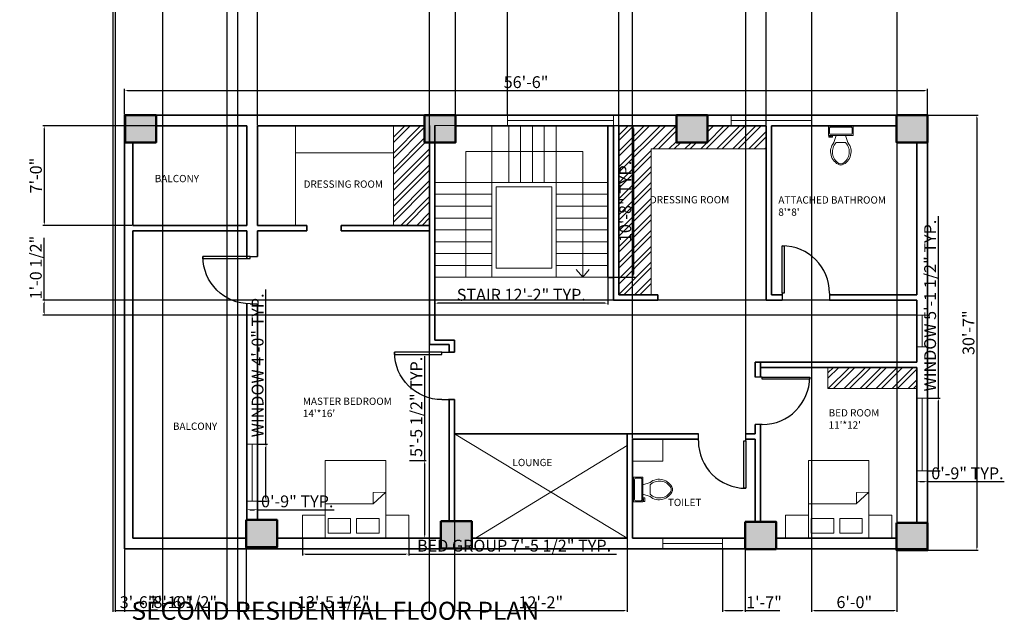
# Model space of a CAD drawing. Units: inches. Extents: x 1964 to 3462, y 1879 to 2909.
# Tile 2 of 4: x 2631 to 3462, y 1879 to 2387. Entities that reach past the tile are written whole.
import ezdxf

# ---------------------------------------------------------------- set-up
doc = ezdxf.new("R2010")
doc.units = ezdxf.units.IN
for name, color, linetype, lineweight in [('A-ANNO-DIMS', 2, 'Continuous', 18), ('A-ANNO-TEXT', 7, 'Continuous', 35), ('A-AREA-IDEN', 7, 'Continuous', 18), ('A-COLS', 1, 'Continuous', 50), ('A-COLS-PATT', 252, 'Continuous', 13), ('A-DOOR', 4, 'Continuous', 25), ('A-FLOR-CASE', 9, 'Continuous', 18), ('A-FLOR-FIXT', 4, 'Continuous', 18), ('A-FLOR-OPEN', 8, 'Continuous', 13), ('A-FLOR-PATT', 252, 'Continuous', 13), ('A-FLOR-STRS', 3, 'Continuous', 18), ('A-FURN', 8, 'Continuous', 18), ('A-GLAZ', 4, 'Continuous', 18), ('A-WALL', 7, 'Continuous', 35)]:
    doc.layers.add(name, color=color, linetype=linetype, lineweight=lineweight)
doc.styles.get("Standard").update_dxf_attribs({"font": 'arial.ttf'})
doc.dimstyles.new('ISO-25', dxfattribs={"dimtxt": 10, "dimasz": 2.5, "dimexe": 1.25, "dimexo": 0.625, "dimtad": 1, "dimdec": 0, "dimlunit": 4, "dimtxsty": 'Standard', "dimcen": 2.5, "dimadec": 0, "dimazin": 0, "dimtfac": 1, "dimtdec": 0, "dimtmove": 0, "dimatfit": 3, "dimfxl": 1, "dimarcsym": 0})

# ---------------------------------------------------------------- blocks, each defined once
blk = doc.blocks.new('*U2')
for p, q in [((0, 0), (0, -6)), ((40, 0), (40, -6))]:
    blk.add_line(p, q)
blk.add_lwpolyline([(0, 0), (0, 40), (1.75, 40), (1.75, 0)], close=True)
blk.add_arc((0, 0), 40, 0, 90)
blk = doc.blocks.new('*U6')
for p, q in [((-8, -8.5), (-8, -8)), ((-7, -8), (-7, -9.5)), ((-4, -8), (-6, -14)), ((4, -8), (6, -14)), ((9.5, -6), (9.5, -2)), ((-10, -8.5), (-8, -8.5)), ((-10, -9.5), (-10, -8.5)), ((-7, -9.5), (-10, -9.5)), ((4, -14), (-4, -14))]:
    blk.add_line(p, q)
blk.add_lwpolyline([(10.5, -8), (10.5, 0), (-10.5, 0), (-10.5, -8)], close=True)
for points in [[(-9.5, -2), (-9.5, -6)], [(8.5, -1), (-8.5, -1)], [(-8.5, -7), (8.5, -7)]]:
    blk.add_lwpolyline(points)
for centre, radius, start, end in [((-8.62, -1.88), 0.884, 81.8699, 188.1301), ((-8.62, -6.12), 0.884, 171.8699, 278.1301), ((8.62, -1.88), 0.884, 351.8699, 98.1301), ((8.62, -6.12), 0.884, 261.8699, 8.1301), ((3.52, -21.58), 12.17, 141.46911, 247.97143), ((4.2, -21.82), 11.33, 136.36773, 238.94682), ((-3.52, -21.58), 12.17, 292.02843, 38.53071), ((-4.2, -21.82), 11.33, 301.05301, 43.63209), ((0, -27.88), 4, 245.73182, 294.26817), ((0, -29), 4, 254.86053, 285.13947)]:
    blk.add_arc(centre, radius, start, end)
blk = doc.blocks.new('*D11')
at = {"layer": 'A-ANNO-DIMS', "color": 0, "lineweight": -2, "transparency": 16777216}
for p, q in [((2719.86, 2307.2), (2719.86, 2328.6)), ((2722.36, 2327.35), (3395.05, 2327.35)), ((3397.55, 2307.2), (3397.55, 2328.6))]:
    blk.add_line(p, q, dxfattribs=at)
at = {"layer": 'A-ANNO-DIMS', "color": 0, "lineweight": 100, "transparency": 16777216}
for points in [[(2722.36, 2327.76), (2722.36, 2326.93), (2719.86, 2327.35)], [(3395.05, 2327.76), (3395.05, 2326.93), (3397.55, 2327.35)]]:
    blk.add_solid(points, dxfattribs=at)
at = {"layer": 'Defpoints', "color": 0, "lineweight": 100, "transparency": 16777216}
for p in [(3397.55, 2327.35), (2719.86, 2306.57), (3397.55, 2306.57)]:
    blk.add_point(p, dxfattribs=at)
at = {"layer": 'A-ANNO-DIMS', "color": 0, "transparency": 16777216, "insert": (3058.71, 2333.08), "char_height": 10, "attachment_point": 5}
blk.add_mtext('56\'-6"', dxfattribs=at)
blk = doc.blocks.new('*D12')
at = {"layer": 'A-ANNO-DIMS', "color": 0, "lineweight": -2, "transparency": 16777216}
for p, q in [((3398.18, 2306.57), (3440.34, 2306.57)), ((3439.09, 2304.07), (3439.09, 1941.77)), ((3398.18, 1939.27), (3440.34, 1939.27))]:
    blk.add_line(p, q, dxfattribs=at)
at = {"layer": 'A-ANNO-DIMS', "color": 0, "lineweight": 100, "transparency": 16777216}
for points in [[(3438.67, 2304.07), (3439.5, 2304.07), (3439.09, 2306.57)], [(3438.67, 1941.77), (3439.5, 1941.77), (3439.09, 1939.27)]]:
    blk.add_solid(points, dxfattribs=at)
at = {"layer": 'Defpoints', "color": 0, "lineweight": 100, "transparency": 16777216}
for p in [(3397.55, 2306.57), (3397.55, 1939.27), (3439.09, 1939.27)]:
    blk.add_point(p, dxfattribs=at)
at = {"layer": 'A-ANNO-DIMS', "color": 0, "transparency": 16777216, "insert": (3433.35, 2122.92), "char_height": 10, "attachment_point": 5, "rotation": 90}
blk.add_mtext('30\'-7"', dxfattribs=at)
blk = doc.blocks.new('COL-RECT-26x23')
blk.add_lwpolyline([(0, 23.08), (26.15, 23.08), (26.15, 0), (0, 0)], close=True)
blk = doc.blocks.new('BED-DOUBLE-WITH-NIGHTSTANDS')
for p, q in [((59.67, 28.98), (70.38, 38.71)), ((70.38, 38.71), (59.8, 38.58)), ((59.8, 38.58), (59.8, 29.09)), ((19.34, 28.98), (59.67, 28.98))]:
    blk.add_line(p, q)
for points in [[(19.34, 0), (70.38, 0), (70.38, 65.5), (19.34, 65.5)], [(19.34, 0), (0, 0), (0, 19.34), (19.34, 19.34)], [(89.72, 0), (70.38, 0), (70.38, 19.34), (89.72, 19.34)], [(21.67, 4.3), (40.69, 4.3), (40.69, 16.59), (21.67, 16.59)], [(45.74, 4.3), (64.76, 4.3), (64.76, 16.59), (45.74, 16.59)]]:
    blk.add_lwpolyline(points, close=True)
blk = doc.blocks.new('STAIR-RETURN-RESIDENTIAL')
for p, q in [((0, 128), (145.76, 128)), ((21.08, 128), (15.66, 121.5)), ((21.08, 21.87), (21.08, 128)), ((21.08, 128), (26.5, 121.5)), ((43.5, 124.05), (43.5, 128)), ((97.76, 128), (97.76, 118)), ((119.78, 128), (119.78, 21.87)), ((0, 118), (43.5, 118)), ((43.5, 48), (43.5, 124.05)), ((47.14, 51.64), (47.14, 120.41)), ((47.14, 120.41), (94.12, 120.41)), ((94.12, 51.64), (94.12, 120.41)), ((97.76, 48), (97.76, 124.05)), ((97.76, 118), (145.76, 118)), ((0, 108), (43.5, 108)), ((97.76, 108), (145.76, 108)), ((0, 98), (43.5, 98)), ((97.76, 98), (145.76, 98)), ((0, 88), (43.5, 88)), ((97.76, 88), (145.76, 88)), ((0, 78), (43.5, 78)), ((97.76, 78), (145.76, 78)), ((0, 68), (43.5, 68)), ((97.76, 68), (145.76, 68)), ((0, 58), (43.5, 58)), ((94.12, 51.64), (47.14, 51.64)), ((97.76, 58), (145.76, 58)), ((97.76, 50.18), (97.76, 0)), ((0, 48), (145.76, 48)), ((97.76, 48), (43.5, 48)), ((43.5, 48), (43.5, 0)), ((53.5, 48), (53.5, 0)), ((63.5, 48), (63.5, 0)), ((73.5, 48), (73.5, 0)), ((83.5, 48), (83.5, 0)), ((119.78, 21.87), (21.08, 21.87))]:
    blk.add_line(p, q)
blk = doc.blocks.new('WIN-48IN')
blk.add_line((4.5, 0), (4.5, 48.18))
blk.add_lwpolyline([(0, 0), (9, 0), (9, 48.18), (0, 48.18)], close=True)
blk = doc.blocks.new('WIN-50IN')
blk.add_line((0, 4.5), (50.22, 4.5))
blk.add_lwpolyline([(0, 9), (50.22, 9), (50.22, 0), (0, 0)], close=True)
blk = doc.blocks.new('WIN-61IN')
blk.add_line((4.5, 61.35), (4.5, 0))
blk.add_lwpolyline([(0, 61.35), (9, 61.35), (9, 0), (0, 0)], close=True)
blk = doc.blocks.new('WIN-27IN')
blk.add_line((4.5, 26.51), (4.5, 0))
blk.add_lwpolyline([(0, 0), (9, 0), (9, 26.51), (0, 26.51)], close=True)
blk = doc.blocks.new('WIN-90IN')
blk.add_line((0, 4.5), (89.57, 4.5))
blk.add_lwpolyline([(0, 9), (89.57, 9), (89.57, 0), (0, 0)], close=True)
blk = doc.blocks.new('*D29')
at = {"layer": 'A-ANNO-DIMS', "color": 0, "lineweight": -2, "transparency": 16777216}
for p, q in [((2870.02, 1948.95), (2870.02, 1934.86)), ((2959.73, 1948.95), (2959.73, 1934.86)), ((2872.52, 1936.11), (2957.23, 1936.11)), ((2959.73, 1936.11), (3135.01, 1936.11))]:
    blk.add_line(p, q, dxfattribs=at)
at = {"layer": 'A-ANNO-DIMS', "color": 0, "lineweight": 100, "transparency": 16777216}
for points in [[(2872.52, 1936.53), (2872.52, 1935.7), (2870.02, 1936.11)], [(2957.23, 1936.53), (2957.23, 1935.7), (2959.73, 1936.11)]]:
    blk.add_solid(points, dxfattribs=at)
at = {"layer": 'Defpoints', "color": 0, "lineweight": 100, "transparency": 16777216}
for p in [(2870.02, 1949.57), (2959.73, 1949.57), (2959.73, 1936.11)]:
    blk.add_point(p, dxfattribs=at)
at = {"layer": 'A-ANNO-DIMS', "color": 0, "transparency": 16777216, "insert": (3048.62, 1941.91), "char_height": 10, "attachment_point": 5}
blk.add_mtext('BED GROUP 7\'-5 1/2" TYP.', dxfattribs=at)
blk = doc.blocks.new('*D30')
at = {"layer": 'A-ANNO-DIMS', "color": 0, "lineweight": -2, "transparency": 16777216}
for p, q in [((2973.19, 2015.07), (2973.19, 2103.08)), ((2960.36, 2015.07), (2974.44, 2015.07)), ((2973.19, 1952.07), (2973.19, 2012.57)), ((2960.36, 1949.57), (2974.44, 1949.57))]:
    blk.add_line(p, q, dxfattribs=at)
at = {"layer": 'A-ANNO-DIMS', "color": 0, "lineweight": 100, "transparency": 16777216}
for points in [[(2972.77, 2012.57), (2973.61, 2012.57), (2973.19, 2015.07)], [(2972.77, 1952.07), (2973.61, 1952.07), (2973.19, 1949.57)]]:
    blk.add_solid(points, dxfattribs=at)
at = {"layer": 'Defpoints', "color": 0, "lineweight": 100, "transparency": 16777216}
for p in [(2959.73, 2015.07), (2973.19, 2015.07), (2959.73, 1949.57)]:
    blk.add_point(p, dxfattribs=at)
at = {"layer": 'A-ANNO-DIMS', "color": 0, "transparency": 16777216, "insert": (2967.39, 2060.33), "char_height": 10, "attachment_point": 5, "rotation": 90}
blk.add_mtext('5\'-5 1/2" TYP.', dxfattribs=at)
blk = doc.blocks.new('*D31')
at = {"layer": 'A-ANNO-DIMS', "color": 0, "lineweight": -2, "transparency": 16777216}
for p, q in [((2981.84, 2169.09), (2981.84, 2146.6)), ((3127.6, 2169.09), (3127.6, 2146.6)), ((3125.1, 2147.85), (2984.34, 2147.85))]:
    blk.add_line(p, q, dxfattribs=at)
at = {"layer": 'A-ANNO-DIMS', "color": 0, "lineweight": 100, "transparency": 16777216}
for points in [[(2984.34, 2148.27), (2984.34, 2147.43), (2981.84, 2147.85)], [(3125.1, 2148.27), (3125.1, 2147.43), (3127.6, 2147.85)]]:
    blk.add_solid(points, dxfattribs=at)
at = {"layer": 'Defpoints', "color": 0, "lineweight": 100, "transparency": 16777216}
for p in [(2981.84, 2169.71), (3127.6, 2169.71), (2981.84, 2147.85)]:
    blk.add_point(p, dxfattribs=at)
at = {"layer": 'A-ANNO-DIMS', "color": 0, "transparency": 16777216, "insert": (3054.72, 2153.65), "char_height": 10, "attachment_point": 5}
blk.add_mtext('STAIR 12\'-2" TYP.', dxfattribs=at)
blk = doc.blocks.new('*D32')
at = {"layer": 'A-ANNO-DIMS', "color": 0, "lineweight": -2, "transparency": 16777216}
for p, q in [((3128.22, 2297.71), (3150.71, 2297.71)), ((3149.46, 2295.21), (3149.46, 2172.21)), ((3128.22, 2169.71), (3150.71, 2169.71))]:
    blk.add_line(p, q, dxfattribs=at)
at = {"layer": 'A-ANNO-DIMS', "color": 0, "lineweight": 100, "transparency": 16777216}
for points in [[(3149.05, 2295.21), (3149.88, 2295.21), (3149.46, 2297.71)], [(3149.05, 2172.21), (3149.88, 2172.21), (3149.46, 2169.71)]]:
    blk.add_solid(points, dxfattribs=at)
at = {"layer": 'Defpoints', "color": 0, "lineweight": 100, "transparency": 16777216}
for p in [(3127.6, 2297.71), (3127.6, 2169.71), (3149.46, 2169.71)]:
    blk.add_point(p, dxfattribs=at)
at = {"layer": 'A-ANNO-DIMS', "color": 0, "transparency": 16777216, "insert": (3143.73, 2233.71), "char_height": 10, "attachment_point": 5, "rotation": 90}
blk.add_mtext('10\'-8" TYP.', dxfattribs=at)
blk = doc.blocks.new('*D33')
at = {"layer": 'A-ANNO-DIMS', "color": 0, "lineweight": -2, "transparency": 16777216}
for p, q in [((2839.29, 2028.96), (2839.29, 2159.25)), ((2832.69, 2028.96), (2840.54, 2028.96)), ((2839.29, 1983.28), (2839.29, 2026.46)), ((2832.69, 1980.78), (2840.54, 1980.78))]:
    blk.add_line(p, q, dxfattribs=at)
at = {"layer": 'A-ANNO-DIMS', "color": 0, "lineweight": 100, "transparency": 16777216}
for points in [[(2838.88, 2026.46), (2839.71, 2026.46), (2839.29, 2028.96)], [(2838.88, 1983.28), (2839.71, 1983.28), (2839.29, 1980.78)]]:
    blk.add_solid(points, dxfattribs=at)
at = {"layer": 'Defpoints', "color": 0, "lineweight": 100, "transparency": 16777216}
for p in [(2832.07, 2028.96), (2839.29, 2028.96), (2832.07, 1980.78)]:
    blk.add_point(p, dxfattribs=at)
at = {"layer": 'A-ANNO-DIMS', "color": 0, "transparency": 16777216, "insert": (2833.49, 2095.36), "char_height": 10, "attachment_point": 5, "rotation": 90}
blk.add_mtext('WINDOW 4\'-0" TYP.', dxfattribs=at)
blk = doc.blocks.new('*D34')
at = {"layer": 'A-ANNO-DIMS', "color": 0, "lineweight": -2, "transparency": 16777216}
for p, q in [((2823.07, 1980.15), (2823.07, 1972.3)), ((2832.07, 1980.15), (2832.07, 1972.3)), ((2825.57, 1973.55), (2829.57, 1973.55)), ((2832.07, 1973.55), (2896.77, 1973.55))]:
    blk.add_line(p, q, dxfattribs=at)
at = {"layer": 'A-ANNO-DIMS', "color": 0, "lineweight": 100, "transparency": 16777216}
for points in [[(2825.57, 1973.97), (2825.57, 1973.13), (2823.07, 1973.55)], [(2829.57, 1973.97), (2829.57, 1973.13), (2832.07, 1973.55)]]:
    blk.add_solid(points, dxfattribs=at)
at = {"layer": 'Defpoints', "color": 0, "lineweight": 100, "transparency": 16777216}
for p in [(2823.07, 1980.78), (2832.07, 1980.78), (2832.07, 1973.55)]:
    blk.add_point(p, dxfattribs=at)
at = {"layer": 'A-ANNO-DIMS', "color": 0, "transparency": 16777216, "insert": (2865.67, 1979.28), "char_height": 10, "attachment_point": 5}
blk.add_mtext('0\'-9" TYP.', dxfattribs=at)
blk = doc.blocks.new('*D37')
at = {"layer": 'A-ANNO-DIMS', "color": 0, "lineweight": -2, "transparency": 16777216}
for p, q in [((3406.76, 2067.79), (3406.76, 2221.38)), ((3398.18, 2067.79), (3408.01, 2067.79)), ((3406.76, 2008.94), (3406.76, 2065.29)), ((3398.18, 2006.44), (3408.01, 2006.44))]:
    blk.add_line(p, q, dxfattribs=at)
at = {"layer": 'A-ANNO-DIMS', "color": 0, "lineweight": 100, "transparency": 16777216}
for points in [[(3406.34, 2065.29), (3407.17, 2065.29), (3406.76, 2067.79)], [(3406.34, 2008.94), (3407.17, 2008.94), (3406.76, 2006.44)]]:
    blk.add_solid(points, dxfattribs=at)
at = {"layer": 'Defpoints', "color": 0, "lineweight": 100, "transparency": 16777216}
for p in [(3397.55, 2067.79), (3406.76, 2067.79), (3397.55, 2006.44)]:
    blk.add_point(p, dxfattribs=at)
at = {"layer": 'A-ANNO-DIMS', "color": 0, "transparency": 16777216, "insert": (3400.96, 2145.83), "char_height": 10, "attachment_point": 5, "rotation": 90}
blk.add_mtext('WINDOW 5\'-1 1/2" TYP.', dxfattribs=at)
blk = doc.blocks.new('*D38')
at = {"layer": 'A-ANNO-DIMS', "color": 0, "lineweight": -2, "transparency": 16777216}
for p, q in [((3388.55, 2005.81), (3388.55, 1995.98)), ((3397.55, 2005.81), (3397.55, 1995.98)), ((3391.05, 1997.23), (3395.05, 1997.23)), ((3397.55, 1997.23), (3462.26, 1997.23))]:
    blk.add_line(p, q, dxfattribs=at)
at = {"layer": 'A-ANNO-DIMS', "color": 0, "lineweight": 100, "transparency": 16777216}
for points in [[(3391.05, 1997.65), (3391.05, 1996.82), (3388.55, 1997.23)], [(3395.05, 1997.65), (3395.05, 1996.82), (3397.55, 1997.23)]]:
    blk.add_solid(points, dxfattribs=at)
at = {"layer": 'Defpoints', "color": 0, "lineweight": 100, "transparency": 16777216}
for p in [(3388.55, 2006.44), (3397.55, 2006.44), (3397.55, 1997.23)]:
    blk.add_point(p, dxfattribs=at)
at = {"layer": 'A-ANNO-DIMS', "color": 0, "transparency": 16777216, "insert": (3431.16, 2002.96), "char_height": 10, "attachment_point": 5}
blk.add_mtext('0\'-9" TYP.', dxfattribs=at)
blk = doc.blocks.new('*D53')
at = {"layer": 'A-ANNO-DIMS', "color": 0, "lineweight": -2, "transparency": 16777216}
for p, q in [((2709.93, 2826.73), (2709.93, 1887.22)), ((2751.91, 2826.73), (2751.91, 1887.22)), ((2712.43, 1888.47), (2749.41, 1888.47))]:
    blk.add_line(p, q, dxfattribs=at)
at = {"layer": 'A-ANNO-DIMS', "color": 0, "lineweight": 100, "transparency": 16777216}
for points in [[(2712.43, 1888.89), (2712.43, 1888.06), (2709.93, 1888.47)], [(2749.41, 1888.89), (2749.41, 1888.06), (2751.91, 1888.47)]]:
    blk.add_solid(points, dxfattribs=at)
at = {"layer": 'Defpoints', "color": 0, "lineweight": 100, "transparency": 16777216}
for p in [(2709.93, 2827.36), (2751.91, 2827.36), (2751.91, 1888.47)]:
    blk.add_point(p, dxfattribs=at)
at = {"layer": 'A-ANNO-DIMS', "color": 0, "transparency": 16777216, "insert": (2730.92, 1894.21), "char_height": 10, "attachment_point": 5}
blk.add_mtext('3\'-6"', dxfattribs=at)
blk = doc.blocks.new('*D56')
at = {"layer": 'A-ANNO-DIMS', "color": 0, "lineweight": -2, "transparency": 16777216}
for p, q in [((3299.67, 2687.56), (3299.67, 1887.22)), ((3371.67, 2687.56), (3371.67, 1887.22)), ((3302.17, 1888.47), (3369.17, 1888.47))]:
    blk.add_line(p, q, dxfattribs=at)
at = {"layer": 'A-ANNO-DIMS', "color": 0, "lineweight": 100, "transparency": 16777216}
for points in [[(3302.17, 1888.89), (3302.17, 1888.06), (3299.67, 1888.47)], [(3369.17, 1888.89), (3369.17, 1888.06), (3371.67, 1888.47)]]:
    blk.add_solid(points, dxfattribs=at)
at = {"layer": 'Defpoints', "color": 0, "lineweight": 100, "transparency": 16777216}
for p in [(3299.67, 2688.18), (3371.67, 2688.18), (3371.67, 1888.47)]:
    blk.add_point(p, dxfattribs=at)
at = {"layer": 'A-ANNO-DIMS', "color": 0, "transparency": 16777216, "insert": (3335.67, 1894.2), "char_height": 10, "attachment_point": 5}
blk.add_mtext('6\'-0"', dxfattribs=at)
blk = doc.blocks.new('*D57')
at = {"layer": 'A-ANNO-DIMS', "color": 0, "lineweight": -2, "transparency": 16777216}
for p, q in [((2711.98, 2582.23), (2711.98, 1887.22)), ((2806.18, 2582.23), (2806.18, 1887.22)), ((2714.48, 1888.47), (2803.68, 1888.47))]:
    blk.add_line(p, q, dxfattribs=at)
at = {"layer": 'A-ANNO-DIMS', "color": 0, "lineweight": 100, "transparency": 16777216}
for points in [[(2714.48, 1888.89), (2714.48, 1888.06), (2711.98, 1888.47)], [(2803.68, 1888.89), (2803.68, 1888.06), (2806.18, 1888.47)]]:
    blk.add_solid(points, dxfattribs=at)
at = {"layer": 'Defpoints', "color": 0, "lineweight": 100, "transparency": 16777216}
for p in [(2711.98, 2582.86), (2806.18, 2582.86), (2806.18, 1888.47)]:
    blk.add_point(p, dxfattribs=at)
at = {"layer": 'A-ANNO-DIMS', "color": 0, "transparency": 16777216, "insert": (2759.08, 1894.2), "char_height": 10, "attachment_point": 5}
blk.add_mtext('7\'-10"', dxfattribs=at)
blk = doc.blocks.new('*D58')
at = {"layer": 'A-ANNO-DIMS', "color": 0, "lineweight": -2, "transparency": 16777216}
for p, q in [((2815.18, 2582.23), (2815.18, 1887.22)), ((2976.91, 2582.23), (2976.91, 1887.22)), ((2817.68, 1888.47), (2974.41, 1888.47))]:
    blk.add_line(p, q, dxfattribs=at)
at = {"layer": 'A-ANNO-DIMS', "color": 0, "lineweight": 100, "transparency": 16777216}
for points in [[(2817.68, 1888.89), (2817.68, 1888.06), (2815.18, 1888.47)], [(2974.41, 1888.89), (2974.41, 1888.06), (2976.91, 1888.47)]]:
    blk.add_solid(points, dxfattribs=at)
at = {"layer": 'Defpoints', "color": 0, "lineweight": 100, "transparency": 16777216}
for p in [(2815.18, 2582.86), (2976.91, 2582.86), (2976.91, 1888.47)]:
    blk.add_point(p, dxfattribs=at)
at = {"layer": 'A-ANNO-DIMS', "color": 0, "transparency": 16777216, "insert": (2896.05, 1894.27), "char_height": 10, "attachment_point": 5}
blk.add_mtext('13\'-5 1/2"', dxfattribs=at)
blk = doc.blocks.new('*D62')
at = {"layer": 'A-ANNO-DIMS', "color": 0, "lineweight": -2, "transparency": 16777216}
for p, q in [((2719.86, 1939.95), (2719.86, 1887.22)), ((2822.51, 1941.17), (2822.51, 1887.22)), ((2722.36, 1888.47), (2820.01, 1888.47))]:
    blk.add_line(p, q, dxfattribs=at)
at = {"layer": 'A-ANNO-DIMS', "color": 0, "lineweight": 100, "transparency": 16777216}
for points in [[(2722.36, 1888.89), (2722.36, 1888.06), (2719.86, 1888.47)], [(2820.01, 1888.89), (2820.01, 1888.06), (2822.51, 1888.47)]]:
    blk.add_solid(points, dxfattribs=at)
at = {"layer": 'Defpoints', "color": 0, "lineweight": 100, "transparency": 16777216}
for p in [(2719.86, 1940.57), (2822.51, 1941.79), (2822.51, 1888.47)]:
    blk.add_point(p, dxfattribs=at)
at = {"layer": 'A-ANNO-DIMS', "color": 0, "transparency": 16777216, "insert": (2771.18, 1894.27), "char_height": 10, "attachment_point": 5}
blk.add_mtext('8\'-6 1/2"', dxfattribs=at)
blk = doc.blocks.new('*D63')
at = {"layer": 'A-ANNO-DIMS', "color": 0, "lineweight": -2, "transparency": 16777216}
for p, q in [((2745.94, 2297.57), (2650.93, 2297.57)), ((2652.18, 2295.07), (2652.18, 2215.99)), ((2726.19, 2213.49), (2650.93, 2213.49))]:
    blk.add_line(p, q, dxfattribs=at)
at = {"layer": 'A-ANNO-DIMS', "color": 0, "lineweight": 100, "transparency": 16777216}
for points in [[(2651.76, 2295.07), (2652.59, 2295.07), (2652.18, 2297.57)], [(2651.76, 2215.99), (2652.59, 2215.99), (2652.18, 2213.49)]]:
    blk.add_solid(points, dxfattribs=at)
at = {"layer": 'Defpoints', "color": 0, "lineweight": 100, "transparency": 16777216}
for p in [(2746.57, 2297.57), (2652.18, 2213.49), (2726.81, 2213.49)]:
    blk.add_point(p, dxfattribs=at)
at = {"layer": 'A-ANNO-DIMS', "color": 0, "transparency": 16777216, "insert": (2646.45, 2255.53), "char_height": 10, "attachment_point": 5, "rotation": 90}
blk.add_mtext('7\'-0"', dxfattribs=at)
blk = doc.blocks.new('*D64')
at = {"layer": 'A-ANNO-DIMS', "color": 0, "lineweight": -2, "transparency": 16777216}
for p, q in [((2832.07, 2298.2), (2832.07, 2889.94)), ((2834.57, 2888.69), (2974.84, 2888.69)), ((2977.34, 2298.34), (2977.34, 2889.94))]:
    blk.add_line(p, q, dxfattribs=at)
at = {"layer": 'A-ANNO-DIMS', "color": 0, "lineweight": 100, "transparency": 16777216}
for points in [[(2834.57, 2889.1), (2834.57, 2888.27), (2832.07, 2888.69)], [(2974.84, 2889.1), (2974.84, 2888.27), (2977.34, 2888.69)]]:
    blk.add_solid(points, dxfattribs=at)
at = {"layer": 'Defpoints', "color": 0, "lineweight": 100, "transparency": 16777216}
for p in [(2977.34, 2888.69), (2832.07, 2297.57), (2977.34, 2297.71)]:
    blk.add_point(p, dxfattribs=at)
at = {"layer": 'A-ANNO-DIMS', "color": 0, "transparency": 16777216, "insert": (2904.7, 2894.48), "char_height": 10, "attachment_point": 5}
blk.add_mtext('12\'-1 1/2"', dxfattribs=at)
blk = doc.blocks.new('*D65')
at = {"layer": 'A-ANNO-DIMS', "color": 0, "lineweight": -2, "transparency": 16777216}
for p, q in [((3137.07, 2298.2), (3137.07, 2889.94)), ((3139.57, 2888.69), (3258.77, 2888.69)), ((3261.27, 2298.2), (3261.27, 2889.94))]:
    blk.add_line(p, q, dxfattribs=at)
at = {"layer": 'A-ANNO-DIMS', "color": 0, "lineweight": 100, "transparency": 16777216}
for points in [[(3139.57, 2889.1), (3139.57, 2888.27), (3137.07, 2888.69)], [(3258.77, 2889.1), (3258.77, 2888.27), (3261.27, 2888.69)]]:
    blk.add_solid(points, dxfattribs=at)
at = {"layer": 'Defpoints', "color": 0, "lineweight": 100, "transparency": 16777216}
for p in [(3261.27, 2888.69), (3137.07, 2297.57), (3261.27, 2297.57)]:
    blk.add_point(p, dxfattribs=at)
at = {"layer": 'A-ANNO-DIMS', "color": 0, "transparency": 16777216, "insert": (3199.17, 2894.42), "char_height": 10, "attachment_point": 5}
blk.add_mtext('10\'-4"', dxfattribs=at)
blk = doc.blocks.new('*D66')
at = {"layer": 'A-ANNO-DIMS', "color": 0, "lineweight": -2, "transparency": 16777216}
for p, q in [((2998.29, 2037), (2998.29, 1887.22)), ((3144.05, 2037), (3144.05, 1887.22)), ((3000.79, 1888.47), (3141.55, 1888.47))]:
    blk.add_line(p, q, dxfattribs=at)
at = {"layer": 'A-ANNO-DIMS', "color": 0, "lineweight": 100, "transparency": 16777216}
for points in [[(3000.79, 1888.89), (3000.79, 1888.06), (2998.29, 1888.47)], [(3141.55, 1888.89), (3141.55, 1888.06), (3144.05, 1888.47)]]:
    blk.add_solid(points, dxfattribs=at)
at = {"layer": 'Defpoints', "color": 0, "lineweight": 100, "transparency": 16777216}
for p in [(2998.29, 2037.62), (3144.05, 2037.62), (3144.05, 1888.47)]:
    blk.add_point(p, dxfattribs=at)
at = {"layer": 'A-ANNO-DIMS', "color": 0, "transparency": 16777216, "insert": (3071.17, 1894.12), "char_height": 10, "attachment_point": 5}
blk.add_mtext('12\'-2"', dxfattribs=at)
blk = doc.blocks.new('*D67')
at = {"layer": 'A-ANNO-DIMS', "color": 0, "lineweight": -2, "transparency": 16777216}
for p, q in [((3148.55, 2033.75), (3148.55, 2889.94)), ((3151.05, 2888.69), (3241.63, 2888.69)), ((3244.13, 2034), (3244.13, 2889.94))]:
    blk.add_line(p, q, dxfattribs=at)
at = {"layer": 'A-ANNO-DIMS', "color": 0, "lineweight": 100, "transparency": 16777216}
for points in [[(3151.05, 2889.1), (3151.05, 2888.27), (3148.55, 2888.69)], [(3241.63, 2889.1), (3241.63, 2888.27), (3244.13, 2888.69)]]:
    blk.add_solid(points, dxfattribs=at)
at = {"layer": 'Defpoints', "color": 0, "lineweight": 100, "transparency": 16777216}
for p in [(3244.13, 2888.69), (3148.55, 2033.12), (3244.13, 2033.37)]:
    blk.add_point(p, dxfattribs=at)
at = {"layer": 'A-ANNO-DIMS', "color": 0, "transparency": 16777216, "insert": (3196.34, 2894.48), "char_height": 10, "attachment_point": 5}
blk.add_mtext('7\'-11 1/2"', dxfattribs=at)
blk = doc.blocks.new('*D68')
at = {"layer": 'A-ANNO-DIMS', "color": 0, "lineweight": -2, "transparency": 16777216}
for p, q in [((2999.25, 2307.2), (2999.25, 2889.94)), ((3001.75, 2888.69), (3040.51, 2888.69)), ((3043.01, 2307.2), (3043.01, 2889.94))]:
    blk.add_line(p, q, dxfattribs=at)
at = {"layer": 'A-ANNO-DIMS', "color": 0, "lineweight": 100, "transparency": 16777216}
for points in [[(3001.75, 2889.1), (3001.75, 2888.27), (2999.25, 2888.69)], [(3040.51, 2889.1), (3040.51, 2888.27), (3043.01, 2888.69)]]:
    blk.add_solid(points, dxfattribs=at)
at = {"layer": 'Defpoints', "color": 0, "lineweight": 100, "transparency": 16777216}
for p in [(3043.01, 2888.69), (2999.25, 2306.57), (3043.01, 2306.57)]:
    blk.add_point(p, dxfattribs=at)
at = {"layer": 'A-ANNO-DIMS', "color": 0, "transparency": 16777216, "insert": (3021.13, 2894.42), "char_height": 10, "attachment_point": 5}
blk.add_mtext('3\'-8"', dxfattribs=at)
blk = doc.blocks.new('*D69')
at = {"layer": 'A-ANNO-DIMS', "color": 0, "lineweight": -2, "transparency": 16777216}
for p, q in [((3224.47, 1939.95), (3224.47, 1887.22)), ((3243.55, 1939.66), (3243.55, 1887.22)), ((3226.97, 1888.47), (3241.05, 1888.47)), ((3243.55, 1888.47), (3272.95, 1888.47))]:
    blk.add_line(p, q, dxfattribs=at)
at = {"layer": 'A-ANNO-DIMS', "color": 0, "lineweight": 100, "transparency": 16777216}
for points in [[(3226.97, 1888.89), (3226.97, 1888.06), (3224.47, 1888.47)], [(3241.05, 1888.89), (3241.05, 1888.06), (3243.55, 1888.47)]]:
    blk.add_solid(points, dxfattribs=at)
at = {"layer": 'Defpoints', "color": 0, "lineweight": 100, "transparency": 16777216}
for p in [(3224.47, 1940.57), (3243.55, 1940.29), (3243.55, 1888.47)]:
    blk.add_point(p, dxfattribs=at)
at = {"layer": 'A-ANNO-DIMS', "color": 0, "transparency": 16777216, "insert": (3259.5, 1894.12), "char_height": 10, "attachment_point": 5}
blk.add_mtext('1\'-7"', dxfattribs=at)
blk = doc.blocks.new('*D70')
at = {"layer": 'A-ANNO-DIMS', "color": 0, "lineweight": -2, "transparency": 16777216}
for p, q in [((2652.18, 2150.28), (2652.18, 2202.98)), ((3387.93, 2150.28), (2650.93, 2150.28)), ((2652.18, 2140.1), (2652.18, 2147.78)), ((3387.93, 2137.6), (2650.93, 2137.6))]:
    blk.add_line(p, q, dxfattribs=at)
at = {"layer": 'A-ANNO-DIMS', "color": 0, "lineweight": 100, "transparency": 16777216}
for points in [[(2651.76, 2147.78), (2652.59, 2147.78), (2652.18, 2150.28)], [(2651.76, 2140.1), (2652.59, 2140.1), (2652.18, 2137.6)]]:
    blk.add_solid(points, dxfattribs=at)
at = {"layer": 'Defpoints', "color": 0, "lineweight": 100, "transparency": 16777216}
for p in [(2652.18, 2150.28), (3388.55, 2150.28), (3388.55, 2137.6)]:
    blk.add_point(p, dxfattribs=at)
at = {"layer": 'A-ANNO-DIMS', "color": 0, "transparency": 16777216, "insert": (2646.38, 2177.88), "char_height": 10, "attachment_point": 5, "rotation": 90}
blk.add_mtext('1\'-0 1/2"', dxfattribs=at)

msp = doc.modelspace()

# ---------------------------------------------------------------- hatches: boundary and pattern name
at = {"layer": 'A-COLS-PATT'}
h = msp.add_hatch(color=256, dxfattribs=at)
h.dxf.hatch_style = 1
h.paths.add_polyline_path([(3397.55, 2306.57), (3371.4, 2306.57), (3371.4, 2283.49), (3397.55, 2283.49)])
h.paths.add_polyline_path([(3211.73, 2306.57), (3185.58, 2306.57), (3185.58, 2297.57), (3185.79, 2297.57), (3185.79, 2283.49), (3211.73, 2283.49)])
h.paths.add_polyline_path([(2999.25, 2306.57), (2973.1, 2306.57), (2973.1, 2283.49), (2977.89, 2283.49)])
h.paths.add_polyline_path([(2999.25, 2306.57), (2977.89, 2283.49), (2998.29, 2283.49), (2999.25, 2283.49)], flags=17)
h.paths.add_polyline_path([(2746.57, 2306.57), (2720.41, 2306.57), (2745.76, 2283.49), (2746.57, 2283.49)])
h.paths.add_polyline_path([(2720.41, 2306.57), (2720.41, 2283.49), (2745.76, 2283.49)], flags=17)
h.paths.add_polyline_path([(2848.66, 1964.88), (2822.51, 1964.88), (2822.51, 1941.79), (2848.66, 1941.79)])
h.paths.add_polyline_path([(3012.86, 1963.84), (2986.71, 1963.84), (2986.71, 1940.76), (3012.86, 1940.76)])
h.paths.add_polyline_path([(3269.71, 1963.37), (3243.55, 1963.37), (3243.55, 1940.57), (3269.71, 1940.57)])
h.paths.add_polyline_path([(3397.55, 1962.36), (3371.4, 1962.36), (3371.4, 1940.57), (3397.55, 1940.57)])
at = {"layer": 'A-FLOR-PATT'}
h = msp.add_hatch(dxfattribs=at)
h.set_pattern_fill('ANSI32', color=256)
h.set_pattern_definition([(45, (161.698, 257.281), (-6.735192, 6.735192), []), (45, (166.188, 257.281), (-6.735192, 6.735192), [])])
h.paths.add_polyline_path([(3131.67, 2557.57), (3171.89, 2557.57), (3171.89, 2623.36), (3131.67, 2623.36)])
h.paths.add_polyline_path([(3164.38, 2278.1), (3261.27, 2278.1), (3261.27, 2297.57), (3231.68, 2297.57), (3211.73, 2297.57), (3211.73, 2283.49), (3185.58, 2283.49), (3185.58, 2297.57), (3166.29, 2297.57), (3142.29, 2297.57), (3137.07, 2297.57), (3137.07, 2154.78), (3164.38, 2154.78)])
h.paths.add_polyline_path([(2977.34, 2283.49), (2973.1, 2283.49), (2973.1, 2297.57), (2946.77, 2297.57), (2946.77, 2213.49), (2977.34, 2213.49)])
h.paths.add_polyline_path([(3313.48, 2093.57), (3313.48, 2075.7), (3388.55, 2075.7), (3388.55, 2093.57)])
h.paths.add_polyline_path([(3161.01, 2228.59), (3238.21, 2228.59), (3238.21, 2241.28), (3161.01, 2241.28)], flags=24)

# ---------------------------------------------------------------- linework, layer by layer
at = {"layer": 'A-COLS'}
for points in [[(2973.1, 2306.57), (2999.25, 2306.57), (2999.25, 2283.49), (2973.1, 2283.49)], [(3185.58, 2306.57), (3211.73, 2306.57), (3211.73, 2283.49), (3185.58, 2283.49)]]:
    msp.add_lwpolyline(points, close=True, dxfattribs=at)
at = {"layer": 'A-FLOR-CASE'}
for p, q in [((2864.22, 2213.49), (2864.22, 2297.57)), ((2946.77, 2213.49), (2946.77, 2297.57)), ((3164.38, 2154.78), (3164.38, 2278.1)), ((3164.38, 2278.1), (3261.27, 2278.1)), ((2864.22, 2274.77), (2946.77, 2274.77))]:
    msp.add_line(p, q, dxfattribs=at)
msp.add_lwpolyline([(3388.55, 2093.57), (3313.48, 2093.57), (3313.48, 2075.7), (3388.55, 2075.7)], close=True, dxfattribs=at)
at = {"layer": 'A-FLOR-FIXT'}
msp.add_lwpolyline([(3148.55, 2033.12), (3174.08, 2033.12), (3174.08, 2014.52), (3148.55, 2014.52)], close=True, dxfattribs=at)
at = {"layer": 'A-FLOR-OPEN'}
for p, q in [((3144.05, 1949.57), (2998.29, 2037.62)), ((3016.1, 1949.57), (3144.05, 2027.78))]:
    msp.add_line(p, q, dxfattribs=at)
at = {"layer": 'A-FLOR-STRS'}
for q in [(3017.84, 2297.71), (3017.84, 2297.71), (2981.84, 2261.71)]:
    msp.add_line((2981.84, 2297.71), q, dxfattribs=at)
at = {"layer": 'A-GLAZ'}
msp.add_line((3231.68, 2302.07), (3299.86, 2302.07), dxfattribs=at)
msp.add_lwpolyline([(3261.27, 2297.57), (3231.68, 2297.57), (3231.68, 2306.57), (3299.86, 2306.57), (3299.86, 2297.57), (3265.77, 2297.57)], dxfattribs=at)
at = {"layer": 'A-WALL'}
for p, q in [((2768.79, 2306.57), (2719.86, 2306.57)), ((2719.86, 2306.57), (2719.86, 2053.07)), ((2933.79, 2306.57), (2768.79, 2306.57)), ((3397.55, 2306.57), (3397.55, 1940.57)), ((2746.57, 2297.57), (2768.79, 2297.57)), ((2768.79, 2297.57), (2782.83, 2297.57)), ((2777.79, 2297.57), (2823.07, 2297.57)), ((2823.07, 2213.49), (2823.07, 2297.57)), ((2832.07, 2213.49), (2832.07, 2297.57)), ((2832.07, 2297.57), (2973.1, 2297.57)), ((2977.34, 2297.71), (2977.34, 2153.71)), ((2981.84, 2297.71), (2981.84, 2149.21)), ((2999.25, 2297.57), (3132.57, 2297.57)), ((3127.6, 2283.44), (3127.6, 2297.57)), ((3132.57, 2297.57), (3132.57, 2150.28)), ((3137.07, 2297.57), (3137.07, 2154.78)), ((3137.07, 2297.57), (3142.29, 2297.57)), ((3142.29, 2297.57), (3166.29, 2297.57)), ((3166.29, 2297.57), (3185.79, 2297.57)), ((3261.27, 2297.57), (3261.27, 2225.57)), ((3265.77, 2297.57), (3265.77, 2225.57)), ((3371.4, 2297.57), (3316.55, 2297.57)), ((2726.81, 2213.49), (2726.81, 2283.49)), ((3127.6, 2194.21), (3127.6, 2283.44)), ((3261.27, 2225.57), (3261.27, 2150.28)), ((3265.77, 2225.57), (3265.77, 2154.78)), ((2823.07, 2213.49), (2726.81, 2213.49)), ((2873.68, 2213.49), (2832.07, 2213.49)), ((2873.68, 2213.49), (2873.68, 2208.99)), ((2977.34, 2213.49), (2902.74, 2213.49)), ((2902.74, 2213.49), (2902.74, 2208.99)), ((2726.81, 2057.57), (2726.81, 2208.99)), ((2823.07, 2208.99), (2726.81, 2208.99)), ((2823.07, 2185.48), (2823.07, 2208.99)), ((2873.68, 2208.99), (2832.07, 2208.99)), ((2832.07, 2187.23), (2832.07, 2208.99)), ((2977.34, 2208.99), (2902.74, 2208.99)), ((3127.6, 2169.44), (3127.6, 2194.21)), ((3132.1, 2169.44), (3127.6, 2169.44)), ((3132.1, 2169.44), (3132.57, 2169.44)), ((2977.34, 2153.71), (2977.34, 2112.92)), ((3169.87, 2154.78), (3137.07, 2154.78)), ((3169.87, 2154.78), (3169.87, 2150.28)), ((3265.77, 2154.78), (3274.8, 2154.78)), ((3314.8, 2154.78), (3388.55, 2154.78)), ((2823.07, 2053.07), (2823.07, 2147.34)), ((2832.07, 2053.07), (2832.07, 2147.23)), ((2981.84, 2149.21), (2981.84, 2116.62)), ((3169.87, 2150.28), (3132.57, 2150.28)), ((3261.27, 2150.28), (3274.8, 2150.28)), ((3314.8, 2150.28), (3388.55, 2150.28)), ((2993.79, 2112.92), (2977.34, 2112.92)), ((2981.84, 2116.62), (2998.29, 2116.62)), ((2993.79, 2106.51), (2993.79, 2112.92)), ((2998.29, 2116.62), (2998.29, 2106.41)), ((2993.79, 2106.41), (2993.79, 2106.51)), ((2998.29, 2106.41), (2993.79, 2106.41)), ((3388.55, 2098.07), (3252.05, 2098.07)), ((3252.05, 2098.07), (3263.73, 2098.07)), ((3252.05, 2093.57), (3252.05, 2098.07)), ((3256.55, 2093.57), (3256.55, 2098.07)), ((3252.05, 2093.57), (3252.05, 2085.44)), ((3388.55, 2093.57), (3256.55, 2093.57)), ((3256.55, 2093.57), (3256.55, 2085.44)), ((3256.55, 2093.57), (3263.73, 2093.57)), ((3388.55, 1962.36), (3388.55, 2093.57)), ((2998.29, 2066.41), (2993.37, 2066.41)), ((2993.79, 2066.41), (2993.79, 2057.57)), ((2998.29, 2053.07), (2998.29, 2066.41)), ((2719.86, 2053.07), (2719.86, 1940.57)), ((2726.81, 2057.57), (2726.81, 1949.57)), ((2823.07, 2053.07), (2823.07, 1964.88)), ((2832.07, 2053.07), (2832.07, 1964.88)), ((2993.79, 2057.57), (2993.79, 1963.84)), ((2998.29, 2053.07), (2998.29, 1963.84)), ((3252.05, 2045.44), (3252.05, 2037.62)), ((3256.55, 2045.44), (3256.55, 1963.37)), ((3147.39, 2037.62), (2998.29, 2037.62)), ((3144.05, 2037.62), (3144.05, 2025.31)), ((3204.13, 2037.62), (3144.05, 2037.62)), ((3252.05, 2037.62), (3244.13, 2037.62)), ((3144.05, 1949.57), (3144.05, 2027.78)), ((3148.55, 1949.57), (3148.55, 2033.12)), ((3204.13, 2033.12), (3148.55, 2033.12)), ((3252.05, 2033.12), (3244.13, 2033.12)), ((3252.05, 2033.12), (3252.05, 1963.37)), ((3144.05, 1949.57), (3144.05, 1985.57)), ((2726.81, 1949.57), (2789.13, 1949.57)), ((3144.05, 1949.57), (3108.05, 1949.57)), ((3144.05, 1949.57), (3108.05, 1949.57)), ((3180.05, 1949.57), (3148.55, 1949.57)), ((3243.55, 1949.57), (3180.05, 1949.57)), ((2719.86, 1940.57), (2789.13, 1940.57)), ((2768.79, 1940.57), (2881.66, 1940.57))]:
    msp.add_line(p, q, dxfattribs=at)
for points in [[(2768.79, 2306.57), (3397.55, 2306.57), (3397.55, 1940.57), (2768.79, 1940.57)], [(3397.55, 2144.33), (3397.55, 2306.57), (2858.63, 2306.57)], [(2777.79, 2297.57), (2823.07, 2297.57)], [(2832.07, 2297.57), (2973.1, 2297.57)], [(2999.25, 2297.57), (3132.57, 2297.57)], [(3137.07, 2297.57), (3185.79, 2297.57)], [(3211.73, 2297.57), (3261.27, 2297.57)], [(3265.77, 2297.57), (3371.4, 2297.57)], [(3388.55, 2283.49), (3388.55, 2154.78)], [(3388.55, 2150.28), (3388.55, 2098.07)], [(2858.63, 1940.57), (3397.55, 1940.57), (3397.55, 2104.33)], [(3388.55, 2093.57), (3388.55, 1962.36)], [(2823.07, 1949.57), (2777.79, 1949.57)], [(2986.71, 1949.57), (2848.66, 1949.57)], [(3144.05, 1949.57), (3012.86, 1949.57)], [(3243.55, 1949.57), (3148.55, 1949.57)], [(3371.4, 1949.57), (3269.71, 1949.57)]]:
    msp.add_lwpolyline(points, dxfattribs=at)

# ---------------------------------------------------------------- block references
at = {"layer": 'A-COLS'}
for p in [(2720.41, 2283.49), (3371.4, 2283.49), (2822.51, 1941.79), (2986.71, 1940.76), (3243.55, 1940.29), (3371.4, 1939.27)]:
    msp.add_blockref('COL-RECT-26x23', p, dxfattribs=at)
at = {"layer": 'A-DOOR'}
msp.add_blockref('*U2', (3274.8, 2156.28), dxfattribs=at)
at = {"layer": 'A-DOOR', "xscale": -1, "rotation": 90}
for p in [(2826.07, 2187.23), (2987.79, 2106.41)]:
    msp.add_blockref('*U2', p, dxfattribs=at)
at = {"layer": 'A-DOOR'}
for p, rotation in [((3258.05, 2085.44), 270), ((3244.13, 2031.62), 180)]:
    msp.add_blockref('*U2', p, dxfattribs=dict(at, rotation=rotation))
at = {"layer": 'A-FLOR-FIXT'}
msp.add_blockref('*U6', (3324.34, 2297.34), dxfattribs=at)
at = {"layer": 'A-FLOR-FIXT', "rotation": 90}
msp.add_blockref('*U6', (3149.35, 1990.59), dxfattribs=at)
at = {"layer": 'A-FLOR-STRS', "rotation": 180}
msp.add_blockref('STAIR-RETURN-RESIDENTIAL', (3127.6, 2297.71), dxfattribs=at)
at = {"layer": 'A-FURN'}
for p in [(2870.02, 1949.57), (3277.62, 1949.57)]:
    msp.add_blockref('BED-DOUBLE-WITH-NIGHTSTANDS', p, dxfattribs=at)
at = {"layer": 'A-GLAZ'}
for name, p in [('WIN-90IN', (3043.01, 2297.57)), ('WIN-27IN', (3388.56, 2111.09)), ('WIN-61IN', (3388.56, 2006.44)), ('WIN-48IN', (2823.07, 1980.78)), ('WIN-50IN', (3174.25, 1940.57))]:
    msp.add_blockref(name, p, dxfattribs=at)

# ---------------------------------------------------------------- texts
at = {"layer": 'A-ANNO-TEXT', "insert": (2725.78, 1895.87), "char_height": 15.2607, "attachment_point": 1}
msp.add_mtext_dynamic_manual_height_columns('SECOND RESIDENTIAL FLOOR PLAN', width=480.7827, gutter_width=76.3, heights=[0], dxfattribs=at)
at = {"layer": 'A-AREA-IDEN', "attachment_point": 1}
for s, heights, insert, char_height in [('BALCONY', [16.67], (2745.44, 2256.09), 6.161), ('DRESSING ROOM', [0], (2871.03, 2251.41), 6.1611), ('DRESSING ROOM', [0], (3163.21, 2238.22), 6.1611), ("ATTACHED BATHROOM\\P8'*8'", [0], (3271.58, 2238.02), 6.1611), ("MASTER BEDROOM\\P14'*16'", [0], (2870.38, 2068.13), 6.1611), ("BED ROOM\\P11'*12'", [0], (3314.02, 2058.39), 6.161), ('BALCONY', [16.67], (2760.76, 2047.09), 6.161), ('LOUNGE', [0], (3047.24, 2016.46), 6.161), ('TOILET', [0], (3178.38, 1982.77), 6.161)]:
    msp.add_mtext_dynamic_manual_height_columns(s, width=194.1034, gutter_width=30.81, heights=heights, dxfattribs=dict(at, insert=insert, char_height=char_height))

# ---------------------------------------------------------------- dimensions: what is measured, and where the dimension line sits
at = {"layer": 'A-ANNO-DIMS'}
for base, p1, p2, override, picture, middle in [((2977.34, 2888.69), (2832.07, 2297.57), (2977.34, 2297.71), {"dimdec": 1, "dimlfac": 1, "dimrnd": 0, "dimzin": 1, "dimdsep": 46, "dimlunit": 4, "dimfrac": 2}, '*D64', (2904.7, 2894.48)), ((3244.13, 2888.69), (3148.55, 2033.12), (3244.13, 2033.37), {"dimdec": 1, "dimlfac": 1, "dimrnd": 0, "dimzin": 1, "dimdsep": 46, "dimlunit": 4, "dimfrac": 2}, '*D67', (3196.34, 2894.48)), ((3043.01, 2888.69), (2999.25, 2306.57), (3043.01, 2306.57), {"dimdec": 1, "dimlfac": 1, "dimrnd": 0, "dimzin": 1, "dimdsep": 46, "dimlunit": 4, "dimfrac": 2}, '*D68', (3021.13, 2894.42)), ((3261.27, 2888.69), (3137.07, 2297.57), (3261.27, 2297.57), {"dimdec": 1, "dimlfac": 1, "dimrnd": 0, "dimzin": 1, "dimdsep": 46, "dimlunit": 4, "dimfrac": 2}, '*D65', (3199.17, 2894.42)), ((2751.91, 1888.47), (2709.93, 2827.36), (2751.91, 2827.36), {"dimdec": 1, "dimlfac": 1, "dimrnd": 0, "dimzin": 1, "dimdsep": 46, "dimlunit": 4, "dimfrac": 2}, '*D53', (2730.92, 1894.21)), ((3371.67, 1888.47), (3299.67, 2688.18), (3371.67, 2688.18), {"dimdec": 1, "dimlfac": 1, "dimrnd": 0, "dimzin": 1, "dimdsep": 46, "dimlunit": 4, "dimfrac": 2}, '*D56', (3335.67, 1894.2)), ((2806.18, 1888.47), (2711.98, 2582.86), (2806.18, 2582.86), {"dimdec": 1, "dimlfac": 1, "dimrnd": 0, "dimzin": 1, "dimdsep": 46, "dimlunit": 4, "dimfrac": 2}, '*D57', (2759.08, 1894.2)), ((2976.91, 1888.47), (2815.18, 2582.86), (2976.91, 2582.86), {"dimdec": 1, "dimlfac": 1, "dimrnd": 0, "dimzin": 1, "dimdsep": 46, "dimlunit": 4, "dimfrac": 2}, '*D58', (2896.05, 1894.27)), ((3397.55, 2327.35), (2719.86, 2306.57), (3397.55, 2306.57), {"dimclrd": 0, "dimclre": 0, "dimclrt": 0}, '*D11', (3058.71, 2333.08)), ((3144.05, 1888.47), (2998.29, 2037.62), (3144.05, 2037.62), {"dimdec": 1, "dimlfac": 1, "dimrnd": 0, "dimzin": 1, "dimdsep": 46, "dimlunit": 4, "dimfrac": 2}, '*D66', (3071.17, 1894.12)), ((2822.5068, 1888.4735), (2719.8601, 1940.5718), (2822.5068, 1941.7943), {"dimdec": 1, "dimlfac": 1, "dimrnd": 0, "dimzin": 1, "dimdsep": 46, "dimlunit": 4, "dimfrac": 2}, '*D62', (2771.1835, 1894.269)), ((3243.55, 1888.47), (3224.47, 1940.57), (3243.55, 1940.29), {"dimdec": 1, "dimlfac": 1, "dimrnd": 0, "dimzin": 1, "dimdsep": 46, "dimlunit": 4, "dimfrac": 2}, '*D69', (3259.5, 1894.12))]:
    dim = msp.add_linear_dim(base=base, p1=p1, p2=p2, dimstyle='ISO-25', override=override, dxfattribs=at)
    dim.commit()
    dim.dimension.update_dxf_attribs({"geometry": picture, "text_midpoint": middle})
for base, p1, p2, override, picture, middle in [((3439.09, 1939.27), (3397.55, 2306.57), (3397.55, 1939.27), {"dimclrd": 0, "dimclre": 0, "dimclrt": 0}, '*D12', (3433.35, 2122.92)), ((2652.18, 2213.49), (2746.57, 2297.57), (2726.81, 2213.49), {"dimdec": 1, "dimlfac": 1, "dimrnd": 0, "dimzin": 1, "dimdsep": 46, "dimlunit": 4, "dimfrac": 2}, '*D63', (2646.45, 2255.53)), ((2652.18, 2150.28), (3388.55, 2137.6), (3388.55, 2150.28), {"dimdec": 1, "dimlfac": 1, "dimrnd": 0, "dimzin": 1, "dimdsep": 46, "dimlunit": 4, "dimfrac": 2}, '*D70', (2646.38, 2177.88))]:
    dim = msp.add_linear_dim(base=base, p1=p1, p2=p2, angle=90, dimstyle='ISO-25', override=override, dxfattribs=at)
    dim.commit()
    dim.dimension.update_dxf_attribs({"geometry": picture, "text_midpoint": middle})
for base, p1, p2, angle, text, picture, middle in [((3149.46, 2169.71), (3127.6, 2297.71), (3127.6, 2169.71), 270, '<> TYP.', '*D32', (3143.73, 2233.71)), ((3406.7575, 2067.787), (3397.5549, 2006.4363), (3397.5549, 2067.787), 90, 'WINDOW <> TYP.', '*D37', (3400.9586, 2145.8336)), ((2981.84, 2147.85), (3127.6, 2169.71), (2981.84, 2169.71), 180, 'STAIR <> TYP.', '*D31', (3054.72, 2153.65)), ((2839.29, 2028.96), (2832.07, 1980.78), (2832.07, 2028.96), 90, 'WINDOW <> TYP.', '*D33', (2833.49, 2095.36)), ((2973.19, 2015.07), (2959.73, 1949.57), (2959.73, 2015.07), 90, '<> TYP.', '*D30', (2967.39, 2060.33))]:
    dim = msp.add_linear_dim(base=base, p1=p1, p2=p2, angle=angle, text=text, dimstyle='ISO-25', override={"dimdec": 1, "dimlfac": 1, "dimrnd": 0, "dimzin": 1, "dimdsep": 46, "dimlunit": 4, "dimfrac": 2}, dxfattribs=at)
    dim.commit()
    dim.dimension.update_dxf_attribs({"geometry": picture, "text_midpoint": middle})
for base, p1, p2, text, picture, middle in [((3397.55, 1997.23), (3388.55, 2006.44), (3397.55, 2006.44), '<> TYP.', '*D38', (3431.16, 2002.96)), ((2832.07, 1973.55), (2823.07, 1980.78), (2832.07, 1980.78), '<> TYP.', '*D34', (2865.67, 1979.28)), ((2959.73, 1936.11), (2870.02, 1949.57), (2959.73, 1949.57), 'BED GROUP <> TYP.', '*D29', (3048.62, 1941.91))]:
    dim = msp.add_linear_dim(base=base, p1=p1, p2=p2, text=text, dimstyle='ISO-25', override={"dimdec": 1, "dimlfac": 1, "dimrnd": 0, "dimzin": 1, "dimdsep": 46, "dimlunit": 4, "dimfrac": 2}, dxfattribs=at)
    dim.commit()
    dim.dimension.update_dxf_attribs({"geometry": picture, "text_midpoint": middle})

doc.saveas('drawing.dxf')
